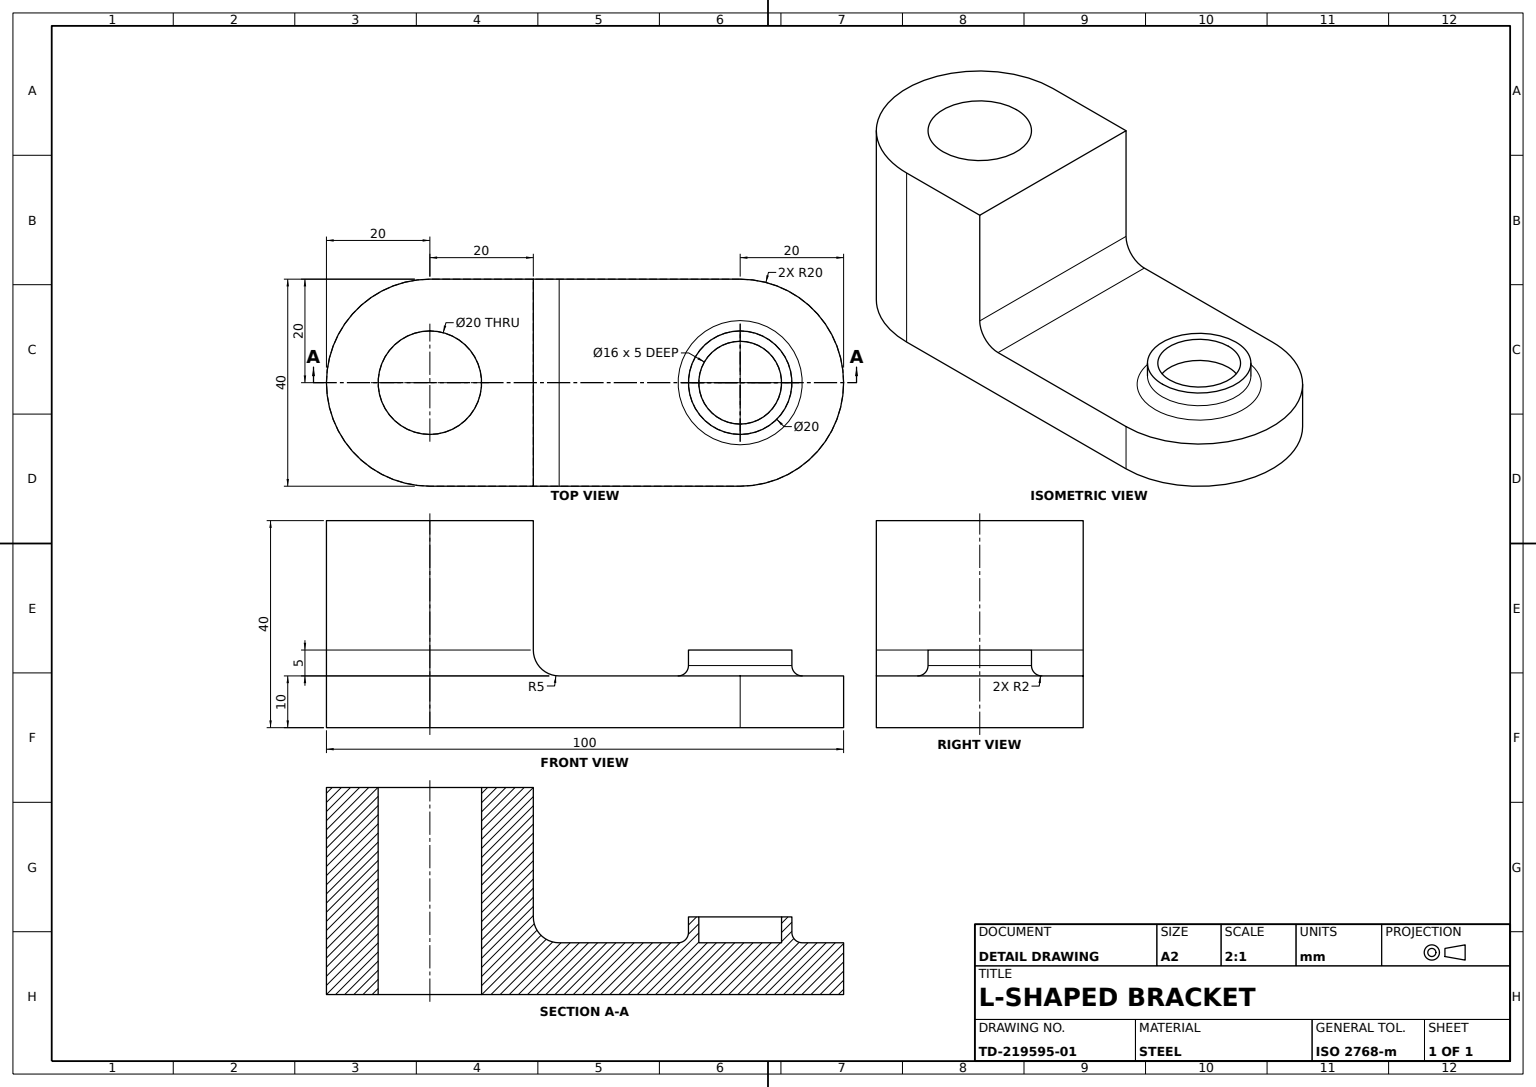
from build123d import *

# Parameters (mm, degrees)
L_BODY_DEPTH               = 40
LUG_END_ROUND_RADIUS       = 20
LUG_END_ROUND_LENGTH       = 40
LUG_BORE_SKETCH_R          = 10
LUG_BORE_20_DEPTH          = 40
BASE_END_ROUND_RADIUS      = 20
BASE_END_ROUND_LENGTH      = 10
RING_BOSS_SKETCH_R         = 10
RING_BOSS_SKETCH_R_2       = 8
RING_BOSS_20X_16_DEPTH     = 5
INNER_CORNER_FILLET_R5_R   = 5
RING_BOSS_BASE_FILLET_R2_R = 2


with BuildPart() as part:
    # L Profile Sketch → L Body (new body)
    with BuildSketch(Plane.XY):
        Polygon((0, 0), (100, 0), (100, 10), (40, 10), (40, 40), (0, 40), align=None)
    extrude(amount=L_BODY_DEPTH)

    # Lug End Round: full round fillet: the end face becomes a half cylinder, R = half its width
    lug_end_round_face = Plane((0, 20, 20), x_dir=(0, 1, 0), z_dir=(-1, 0, 0))  # on the end face: x along it, z out of the body
    lug_end_round_slab = lug_end_round_face.offset(-LUG_END_ROUND_RADIUS / 2) * Box(LUG_END_ROUND_LENGTH, 2 * LUG_END_ROUND_RADIUS, LUG_END_ROUND_RADIUS, mode=Mode.PRIVATE)  # the body's end, R deep
    lug_end_round_round = Plane((20, 20, 20), x_dir=(-1, 0, 0), z_dir=(0, 1, 0)) * Cylinder(LUG_END_ROUND_RADIUS, LUG_END_ROUND_LENGTH, mode=Mode.PRIVATE)  # its axis R under the face
    add(lug_end_round_slab - lug_end_round_round, mode=Mode.SUBTRACT)

    # Lug Bore Sketch → Lug Bore _20 (cut)
    with BuildSketch(Plane(origin=(0, 40, 0), x_dir=(1, 0, 0), z_dir=(0, 1, 0))):
        with Locations(Location((20, -20, 0), (0, 0, 270))):
            Circle(LUG_BORE_SKETCH_R)
    extrude(amount=-LUG_BORE_20_DEPTH, mode=Mode.SUBTRACT)

    # Base End Round: full round fillet: the end face becomes a half cylinder, R = half its width
    base_end_round_face = Plane((100, 5, 20), x_dir=(0, -1, 0), z_dir=(1, 0, 0))  # on the end face: x along it, z out of the body
    base_end_round_slab = base_end_round_face.offset(-BASE_END_ROUND_RADIUS / 2) * Box(BASE_END_ROUND_LENGTH, 2 * BASE_END_ROUND_RADIUS, BASE_END_ROUND_RADIUS, mode=Mode.PRIVATE)  # the body's end, R deep
    base_end_round_round = Plane((80, 5, 20), x_dir=(1, 0, 0), z_dir=(0, -1, 0)) * Cylinder(BASE_END_ROUND_RADIUS, BASE_END_ROUND_LENGTH, mode=Mode.PRIVATE)  # its axis R under the face
    add(base_end_round_slab - base_end_round_round, mode=Mode.SUBTRACT)

    # Ring Boss Sketch → Ring Boss _20x_16 (add)
    with BuildSketch(Plane(origin=(0, 10, 0), x_dir=(1, 0, 0), z_dir=(0, 1, 0))):
        with Locations(Location((80, -20, 0), (0, 0, 90))):
            Circle(RING_BOSS_SKETCH_R)
        with Locations(Location((80, -20, 0), (0, 0, 270))):
            Circle(RING_BOSS_SKETCH_R_2, mode=Mode.SUBTRACT)
    extrude(amount=RING_BOSS_20X_16_DEPTH)

    # Inner Corner Fillet R5
    inner_corner_fillet_r5_edges = [part.edges().sort_by_distance(p)[0] for p in [
        (40, 10, 20),
    ]]
    fillet(inner_corner_fillet_r5_edges, radius=INNER_CORNER_FILLET_R5_R)

    # Ring Boss Base Fillet R2
    ring_boss_base_fillet_r2_edges = [part.edges().sort_by_distance(p)[0] for p in [
        (80, 10, 30),
    ]]
    fillet(ring_boss_base_fillet_r2_edges, radius=RING_BOSS_BASE_FILLET_R2_R)


solid = part.part
